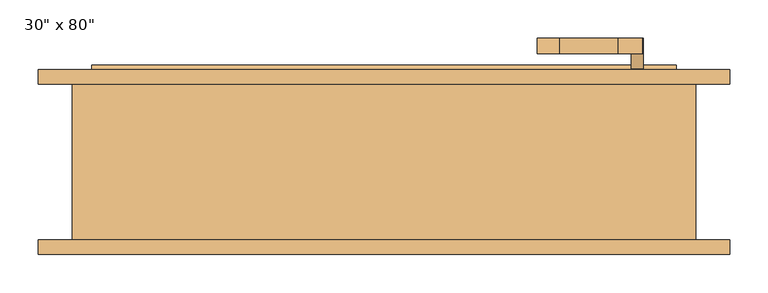
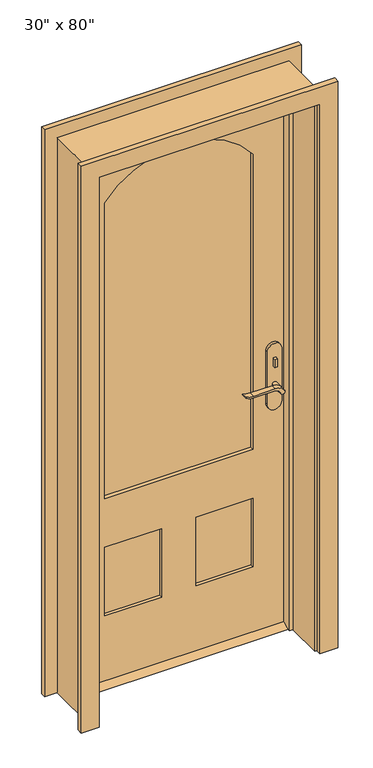
"""IFC4 building model written with IfcOpenShell, lengths in millimetres: door geometry."""

from ifc_helpers import new_model, si_unit, point, frame, frame_2d, origin, place, context, project, spatial, polyline, circle_curve, trimmed, segment, composite_curve, outline, extrude, faceted_brep, source, transform, mapped, element, save


def door_ad59dcae(model_context):
    return source(origin(), model_context, "Body", "SolidModel", [
        extrude(outline(polyline([(63.5, 12.7), (98.425, 12.7), (123.825, 0.0), (38.1, 0.0), (63.5, 12.7)])), frame((-381.0, 0.0, 0.0), z_axis=(1.0, 0.0, 0.0), x_axis=(0.0, 1.0, 0.0)), (0.0, 0.0, 1.0), 762.0),
        extrude(outline(polyline([(335.2, 43.5), (325.2, 43.5), (325.2, 53.5), (335.2, 53.5), (335.2, 43.5)])), frame((0.0, 0.0, 981.9), z_axis=(0.0, 0.0, 1.0), x_axis=(1.0, 0.0, 0.0)), (0.0, 0.0, 1.0), 30.0),
        extrude(outline(composite_curve([segment(trimmed(circle_curve(frame_2d((996.9, 330.2)), 8.0), [point((996.9, 322.2))], [point((996.9, 338.2))], False, "CARTESIAN"), True, "CONTINUOUS"), segment(trimmed(circle_curve(frame_2d((996.9, 330.2)), 8.0), [point((996.9, 338.2))], [point((996.9, 322.2))], False, "CARTESIAN"), True, "CONTINUOUS")], self_intersect=False)), frame((0.0, 108.425, 0.0), z_axis=(0.0, 1.0, 0.0), x_axis=(0.0, 0.0, 1.0)), (0.0, 0.0, 1.0), 10.0),
        extrude(outline(composite_curve([segment(trimmed(circle_curve(frame_2d((897.1555521, 306.5324871)), 37.2832219), [point((919.0523287, 336.7081363))], [point((934.4, 304.8325667))], False, "CARTESIAN"), True, "CONTINUOUS"), segment(polyline([(934.4, 304.8325667), (934.4, 228.5564091)]), True, "CONTINUOUS"), segment(trimmed(circle_curve(frame_2d((1017.6850638, 228.6227909)), 83.2850902), [point((934.4, 228.5564091))], [point((939.4, 200.2))], True, "CARTESIAN"), True, "CONTINUOUS"), segment(polyline([(939.4, 200.2), (936.6135558, 200.2)]), True, "CONTINUOUS"), segment(trimmed(circle_curve(frame_2d((986.6709207, 232.1396612)), 59.3791355), [point((936.6135558, 200.2))], [point((927.4, 228.5564091))], False, "CARTESIAN"), True, "CONTINUOUS"), segment(polyline([(927.4, 228.5564091), (927.4, 304.8138099)]), True, "CONTINUOUS"), segment(trimmed(circle_curve(frame_2d((909.2738613, 304.8138099)), 18.1261387), [point((927.4, 304.8138099))], [point((914.4, 322.2))], True, "CARTESIAN"), True, "CONTINUOUS"), segment(trimmed(circle_curve(frame_2d((914.4, 330.2)), 8.0), [point((914.4, 322.2))], [point((919.0523287, 336.7081363))], False, "CARTESIAN"), True, "CONTINUOUS")], self_intersect=False)), frame((0.0, 3.5, 0.0), z_axis=(0.0, 1.0, 0.0), x_axis=(0.0, 0.0, 1.0)), (0.0, 0.0, 1.0), 20.0),
        extrude(outline(composite_curve([segment(trimmed(circle_curve(frame_2d((914.4, 330.2)), 8.0), [point((914.3999903, 322.2))], [point((919.0523287, 336.7081363))], False, "CARTESIAN"), True, "CONTINUOUS"), segment(trimmed(circle_curve(frame_2d((897.1555521, 306.5324871)), 37.2832219), [point((919.0523287, 336.7081363))], [point((934.4, 304.8325667))], False, "CARTESIAN"), True, "CONTINUOUS"), segment(polyline([(934.4, 304.8325667), (934.4, 228.5564091)]), True, "CONTINUOUS"), segment(trimmed(circle_curve(frame_2d((1017.6850638, 228.6227909)), 83.2850902), [point((934.4, 228.5564091))], [point((939.4, 200.2))], True, "CARTESIAN"), True, "CONTINUOUS"), segment(polyline([(939.4, 200.2), (936.6135558, 200.2)]), True, "CONTINUOUS"), segment(trimmed(circle_curve(frame_2d((986.6709207, 232.1396612)), 59.3791355), [point((936.6135558, 200.2))], [point((927.4, 228.5564091))], False, "CARTESIAN"), True, "CONTINUOUS"), segment(polyline([(927.4, 228.5564091), (927.4, 304.8138122)]), True, "CONTINUOUS"), segment(trimmed(circle_curve(frame_2d((909.2738682, 304.8138122)), 18.1261318), [point((927.4, 304.8138122))], [point((914.3999903, 322.2))], True, "CARTESIAN"), True, "CONTINUOUS")], self_intersect=False)), frame((0.0, 138.425, 0.0), z_axis=(0.0, 1.0, 0.0), x_axis=(0.0, 0.0, 1.0)), (0.0, 0.0, 1.0), 20.0),
        extrude(outline(composite_curve([segment(trimmed(circle_curve(frame_2d((914.4, 330.2)), 8.0), [point((914.4, 322.2))], [point((914.4, 338.2))], False, "CARTESIAN"), True, "CONTINUOUS"), segment(trimmed(circle_curve(frame_2d((914.4, 330.2)), 8.0), [point((914.4, 338.2))], [point((914.4, 322.2))], False, "CARTESIAN"), True, "CONTINUOUS")], self_intersect=False)), frame((0.0, 23.5, 0.0), z_axis=(0.0, 1.0, 0.0), x_axis=(0.0, 0.0, 1.0)), (0.0, 0.0, 1.0), 30.0),
        extrude(outline(composite_curve([segment(trimmed(circle_curve(frame_2d((914.4, 330.2)), 8.0), [point((914.4, 322.2))], [point((914.4, 338.2))], False, "CARTESIAN"), True, "CONTINUOUS"), segment(trimmed(circle_curve(frame_2d((914.4, 330.2)), 8.0), [point((914.4, 338.2))], [point((914.4, 322.2))], False, "CARTESIAN"), True, "CONTINUOUS")], self_intersect=False)), frame((0.0, 108.425, 0.0), z_axis=(0.0, 1.0, 0.0), x_axis=(0.0, 0.0, 1.0)), (0.0, 0.0, 1.0), 30.0),
        extrude(outline(composite_curve([segment(polyline([(844.4, 355.2), (1039.4, 355.2)]), True, "CONTINUOUS"), segment(trimmed(circle_curve(frame_2d((1039.4, 330.2)), 25.0), [point((1039.4, 355.2))], [point((1039.4, 305.2))], False, "CARTESIAN"), True, "CONTINUOUS"), segment(polyline([(1039.4, 305.2), (844.4, 305.2)]), True, "CONTINUOUS"), segment(trimmed(circle_curve(frame_2d((844.4, 330.2)), 25.0), [point((844.4, 305.2))], [point((844.4, 355.2))], False, "CARTESIAN"), True, "CONTINUOUS")], self_intersect=False)), frame((0.0, 53.5, 0.0), z_axis=(0.0, 1.0, 0.0), x_axis=(0.0, 0.0, 1.0)), (0.0, 0.0, 1.0), 10.0),
        extrude(outline(composite_curve([segment(polyline([(844.4, 355.2), (1039.4, 355.2)]), True, "CONTINUOUS"), segment(trimmed(circle_curve(frame_2d((1039.4, 330.2)), 25.0), [point((1039.4, 355.2))], [point((1039.4, 305.2))], False, "CARTESIAN"), True, "CONTINUOUS"), segment(polyline([(1039.4, 305.2), (844.4, 305.2)]), True, "CONTINUOUS"), segment(trimmed(circle_curve(frame_2d((844.4, 330.2)), 25.0), [point((844.4, 305.2))], [point((844.4, 355.2))], False, "CARTESIAN"), True, "CONTINUOUS")], self_intersect=False)), frame((0.0, 98.425, 0.0), z_axis=(0.0, 1.0, 0.0), x_axis=(0.0, 0.0, 1.0)), (0.0, 0.0, 1.0), 10.0),
        extrude(outline(polyline([(2032.0, -381.0), (12.7, -381.0), (12.7, 381.0), (2032.0, 381.0), (2032.0, -381.0)]), holes=[composite_curve([segment(polyline([(688.975, -260.35), (1784.35, -260.35)]), True, "CONTINUOUS"), segment(trimmed(circle_curve(frame_2d((1580.99125, 0.0)), 330.35875), [point((1784.35, -260.35))], [point((1784.35, 260.35))], True, "CARTESIAN"), True, "CONTINUOUS"), segment(polyline([(1784.35, 260.35), (688.975, 260.35), (688.975, -260.35)]), True, "CONTINUOUS")], self_intersect=False), polyline([(508.0, -60.325), (254.0, -60.325), (254.0, -260.35), (508.0, -260.35), (508.0, -60.325)]), polyline([(508.0, 260.35), (254.0, 260.35), (254.0, 60.325), (508.0, 60.325), (508.0, 260.35)])]), frame((0.0, 63.5, 0.0), z_axis=(0.0, 1.0, 0.0), x_axis=(0.0, 0.0, 1.0)), (0.0, 0.0, 1.0), 34.925),
        faceted_brep([(406.4, 98.425, 0.0), (406.4, -104.775, 0.0), (381.0, -104.775, 0.0), (381.0, 28.575, 0.0), (368.3, 28.575, 0.0), (368.3, 63.5, 0.0), (381.0, 63.5, 0.0), (381.0, 98.425, 0.0), (406.4, 98.425, 2057.4), (406.4, -104.775, 2057.4), (-406.4, -104.775, 2057.4), (-406.4, -104.775, 0.0), (-381.0, -104.775, 0.0), (-381.0, -104.775, 2032.0), (381.0, -104.775, 2032.0), (381.0, 28.575, 2032.0), (-381.0, 28.575, 2032.0), (-381.0, 28.575, 0.0), (-368.3, 28.575, 0.0), (-368.3, 28.575, 2019.3), (368.3, 28.575, 2019.3), (368.3, 63.5, 2019.3), (-368.3, 63.5, 2019.3), (-368.3, 63.5, 0.0), (-381.0, 63.5, 0.0), (-381.0, 63.5, 2032.0), (381.0, 63.5, 2032.0), (381.0, 98.425, 2032.0), (-381.0, 98.425, 2032.0), (-381.0, 98.425, 0.0), (-406.4, 98.425, 0.0), (-406.4, 98.425, 2057.4)], [[[0, 1, 2, 3, 4, 5, 6, 7]], [[1, 0, 8, 9]], [[2, 1, 9, 10, 11, 12, 13, 14]], [[3, 2, 14, 15]], [[4, 3, 15, 16, 17, 18, 19, 20]], [[5, 4, 20, 21]], [[6, 5, 21, 22, 23, 24, 25, 26]], [[7, 6, 26, 27]], [[0, 7, 27, 28, 29, 30, 31, 8]], [[9, 8, 31, 10]], [[15, 14, 13, 16]], [[21, 20, 19, 22]], [[27, 26, 25, 28]], [[30, 29, 24, 23, 18, 17, 12, 11]], [[10, 31, 30, 11]], [[16, 13, 12, 17]], [[22, 19, 18, 23]], [[28, 25, 24, 29]]]),
        extrude(outline(polyline([(-60.325, 75.1416667), (-260.35, 75.1416667), (-260.35, 86.7833333), (-60.325, 86.7833333), (-60.325, 75.1416667)])), frame((0.0, 0.0, 254.0), z_axis=(0.0, 0.0, 1.0), x_axis=(1.0, 0.0, 0.0)), (0.0, 0.0, 1.0), 254.0),
        extrude(outline(polyline([(260.35, 75.1416667), (60.325, 75.1416667), (60.325, 86.7833333), (260.35, 86.7833333), (260.35, 75.1416667)])), frame((0.0, 0.0, 254.0), z_axis=(0.0, 0.0, 1.0), x_axis=(1.0, 0.0, 0.0)), (0.0, 0.0, 1.0), 254.0),
        extrude(outline(composite_curve([segment(polyline([(688.975, -260.35), (688.975, 260.35), (1784.35, 260.35)]), True, "CONTINUOUS"), segment(trimmed(circle_curve(frame_2d((1580.99125, 0.0)), 330.35875), [point((1784.35, 260.35))], [point((1784.35, -260.35))], False, "CARTESIAN"), True, "CONTINUOUS"), segment(polyline([(1784.35, -260.35), (688.975, -260.35)]), True, "CONTINUOUS")], self_intersect=False)), frame((0.0, 77.47, 0.0), z_axis=(0.0, 1.0, 0.0), x_axis=(0.0, 0.0, 1.0)), (0.0, 0.0, 1.0), 6.985),
        extrude(outline(polyline([(0.0, -450.85), (0.0, -387.35), (2038.35, -387.35), (2038.35, 387.35), (0.0, 387.35), (0.0, 450.85), (2101.85, 450.85), (2101.85, -450.85), (0.0, -450.85)])), frame((0.0, -123.825, 0.0), z_axis=(0.0, 1.0, 0.0), x_axis=(0.0, 0.0, 1.0)), (0.0, 0.0, 1.0), 19.05),
        extrude(outline(polyline([(0.0, -450.85), (0.0, -387.35), (2038.35, -387.35), (2038.35, 387.35), (0.0, 387.35), (0.0, 450.85), (2101.85, 450.85), (2101.85, -450.85), (0.0, -450.85)])), frame((0.0, 98.425, 0.0), z_axis=(0.0, 1.0, 0.0), x_axis=(0.0, 0.0, 1.0)), (0.0, 0.0, 1.0), 19.05),
    ])


if __name__ == "__main__":
    model = new_model("IFC4")
    model_context = context("Model", 3, world=origin())
    ifc_project = project(units=[si_unit("LENGTHUNIT", "METRE", prefix="MILLI")], contexts=[model_context])
    site = spatial("IfcSite", under=ifc_project)
    building = spatial("IfcBuilding", under=site)
    placement = place(None, origin())
    door_shape = door_ad59dcae(model_context)
    element("IfcDoor", 1, ObjectType="30\" x 80\"", at=placement, inside=building, context=model_context, shape_type="MappedRepresentation", body=[
        mapped(door_shape, transform((0.0, 0.0, 0.0), x_axis=(1.0, 0.0, 0.0), y_axis=(0.0, 1.0, 0.0), z_axis=(0.0, 0.0, 1.0))),
    ])
    save(model, "model.ifc")

# Revit data of these elements
# Type "30\" x 80\""
#   Type Mark = "9"
#   Assembly Code = "B2030100"
#   Analytic Construction = "French door, wood frame with single glass"
#   Threshold Offset [instance default] = 0' - 0 1/2"
#   Thickness = 0' - 1 3/8"
#   Thermal Resistance (R) = 1.0696 (h·ft²·°F)/BTU
#   Swing Angle [instance default] = 90.00°
#   Stiles = 0' - 4 3/4"
#   Rough Width = 2' - 8"
#   Rough Height = 6' - 9"
#   Radius = 1' - 1.00625"
#   Lock Rail = 0' - 7 1/8"
#   Height = 6' - 8"
#   Width = 2' - 6"
#   Heat Transfer Coefficient (U) = 0.9350 BTU/(h·ft²·°F)
#   Door Offset [instance default] = 0' - 0"
#   Bottom Rail = 0' - 9 1/2"
#   Threshold [instance default] = yes
#   Function = 1
#   Exterior Trim [instance default] = yes
#   Trim Material = Cherry
#   Threshold Material = Cherry
#   Panel Material = Cherry
#   Glazing = Glass
#   Frame Material = Cherry
#   Door Handle Material = Aluminum
#   Visual Light Transmittance = 0
#   Solar Heat Gain Coefficient = 0
#   Wall Closure = (empty or 0)
#   Construction Type = (empty or 0)
# Element 1 (IfcDoor, "30\" x 80\"")
#   Materials on its faces: "Cherry", "Aluminum", "Glass"
# Materials
#   "Cherry": class "Wood", colour RGB 226 177 128, transparency 0, Description = "Prunus Serotina", Cost = 0
#   "Glass": class "Glass", colour RGB 0 128 192, transparency 0.75, Description = "Soda Lime Glass", Cost = 0
#   "Aluminum": class "Metal", colour RGB 247 247 247, transparency 0, Description = "Aluminum 6061", Cost = 0
